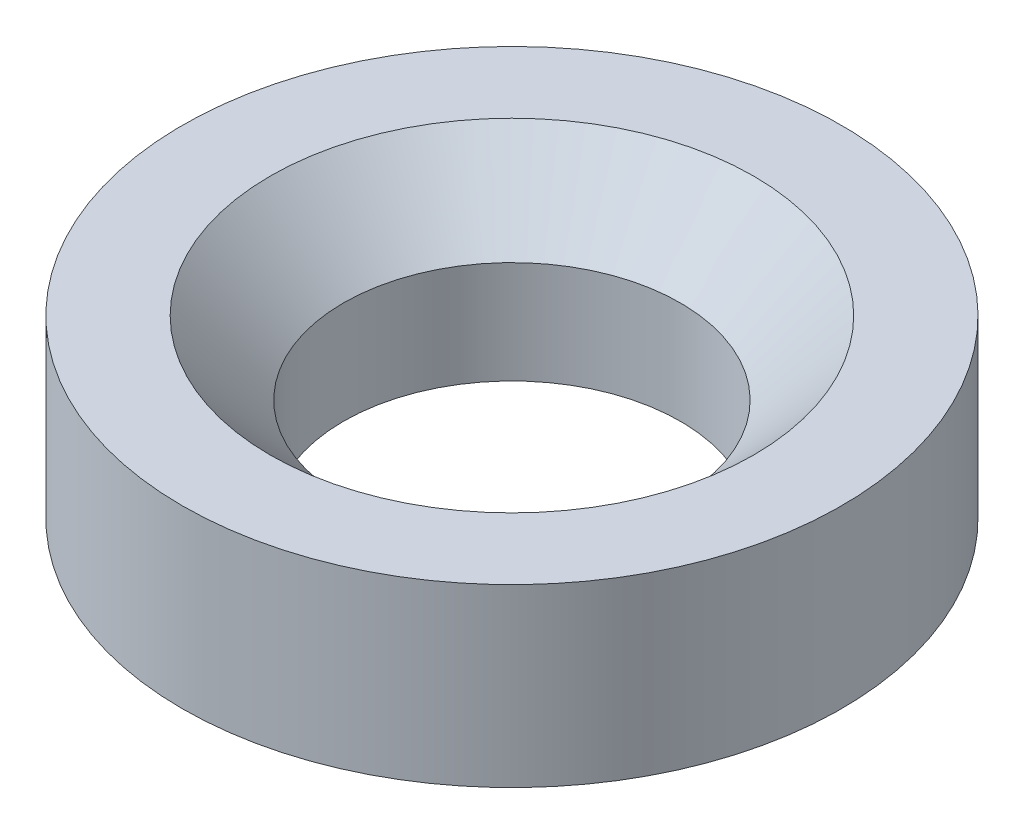
SolidWorks part; units mm, degrees
material "Plain Carbon Steel"
ref_plane "Front Plane" through (0, 0, 0) normal (0, 0, 1) x (1, 0, 0)
ref_plane "Top Plane" through (0, 0, 0) normal (0, 1, 0) x (1, 0, 0)
ref_plane "Right Plane" through (0, 0, 0) normal (1, 0, 0) x (0, 0, -1)
sketch "Bush OD Profile Ø45" plane through (0, 0, 0) normal (0, 1, 0) x (1, 0, 0)
  circle A0 centre (0, 0) radius 22.5
  dimension "D1" = 45
extrude "Bush Body Ø45x12" add sketch "Bush OD Profile Ø45" along normal blind 12
sketch "Countersunk Bore Profile" plane through (0, 0, 0) normal (0, 0, 1) x (1, 0, 0)
  line L0 (11.5, 0) -> (11.5, 7)
  line L1 (-22.5, 0) -> (22.5, 0) construction
  line L2 (11.5, 7) -> (16.5, 12)
  line L3 (22.5, 12) -> (-22.5, 12) construction
  line L4 (16.5, 12) -> (0, 12)
  line L5 (0, 12) -> (0, 0)
  line L6 (0, 0) -> (11.5, 0)
  dimension "D1" = 11.5
  dimension "D2" = 16.5
  dimension "D3" = 135
revolve "Countersunk Bore" cut sketch "Countersunk Bore Profile" angle 360 about L5
